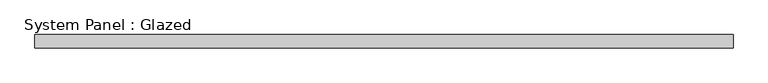
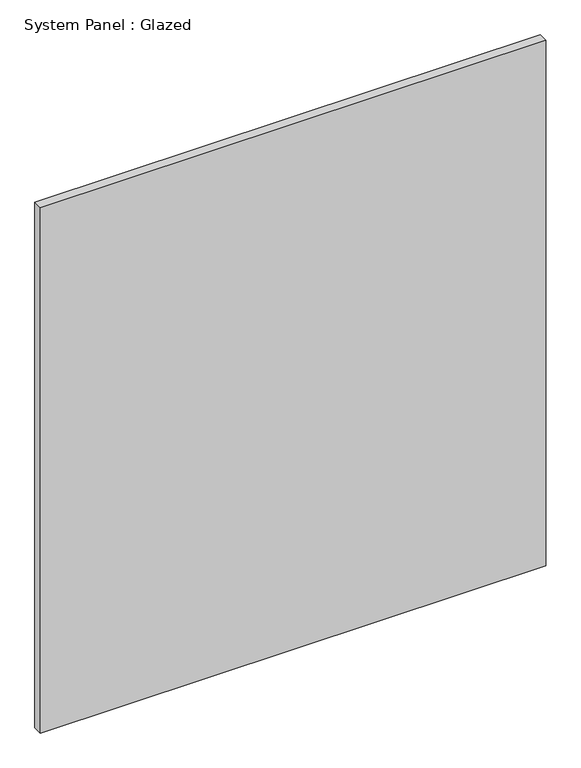
"""IFC4 building model written with IfcOpenShell, lengths in millimetres: plate geometry, System Panel : Glazed."""

from ifc_helpers import new_model, si_unit, origin, origin_with_axes, place, context, project, spatial, polyline, outline, extrude, source, transform, mapped, element, save


def system_panel_glazed_1570095f(model_context):
    return source(origin(), model_context, "Body", "SweptSolid", [
        extrude(outline(polyline([(676.275, 19.05), (-676.275, 19.05), (-676.275, 44.45), (676.275, 44.45), (676.275, 19.05)])), origin_with_axes(), (0.0, 0.0, 1.0), 1486.742764),
    ])


if __name__ == "__main__":
    model = new_model("IFC4")
    model_context = context("Model", 3, world=origin())
    ifc_project = project(units=[si_unit("LENGTHUNIT", "METRE", prefix="MILLI")], contexts=[model_context])
    site = spatial("IfcSite", under=ifc_project)
    building = spatial("IfcBuilding", under=site)
    placement = place(None, origin())
    system_panel_glazed_shape = system_panel_glazed_1570095f(model_context)
    element("IfcPlate", 1, ObjectType="System Panel : Glazed", at=placement, inside=building, context=model_context, shape_type="MappedRepresentation", body=[
        mapped(system_panel_glazed_shape, transform((0.0, 0.0, 0.0), x_axis=(1.0, 0.0, 0.0), y_axis=(0.0, 1.0, 0.0), z_axis=(0.0, 0.0, 1.0))),
    ])
    save(model, "model.ifc")

# Revit data of these elements
# Type "System Panel : Glazed"
#   Construction Type Id = "GSP4R"
#   Analytic Construction = "1/8 in Pilkington single glazing"
#   Visual Light Transmittance = 0.9
#   Solar Heat Gain Coefficient = 0.86
#   Heat Transfer Coefficient (U) = 1.18115 BTU/(h·ft²·°F)
#   Define Thermal Properties by = 1
# Element 1 (IfcPlate, "System Panel : Glazed")
#   Materials on its faces: "Glass"
# Materials
#   "Glass": class "Glass", colour RGB 0 128 192, transparency 0.75, Description = "Soda Lime Glass", Cost = 0
